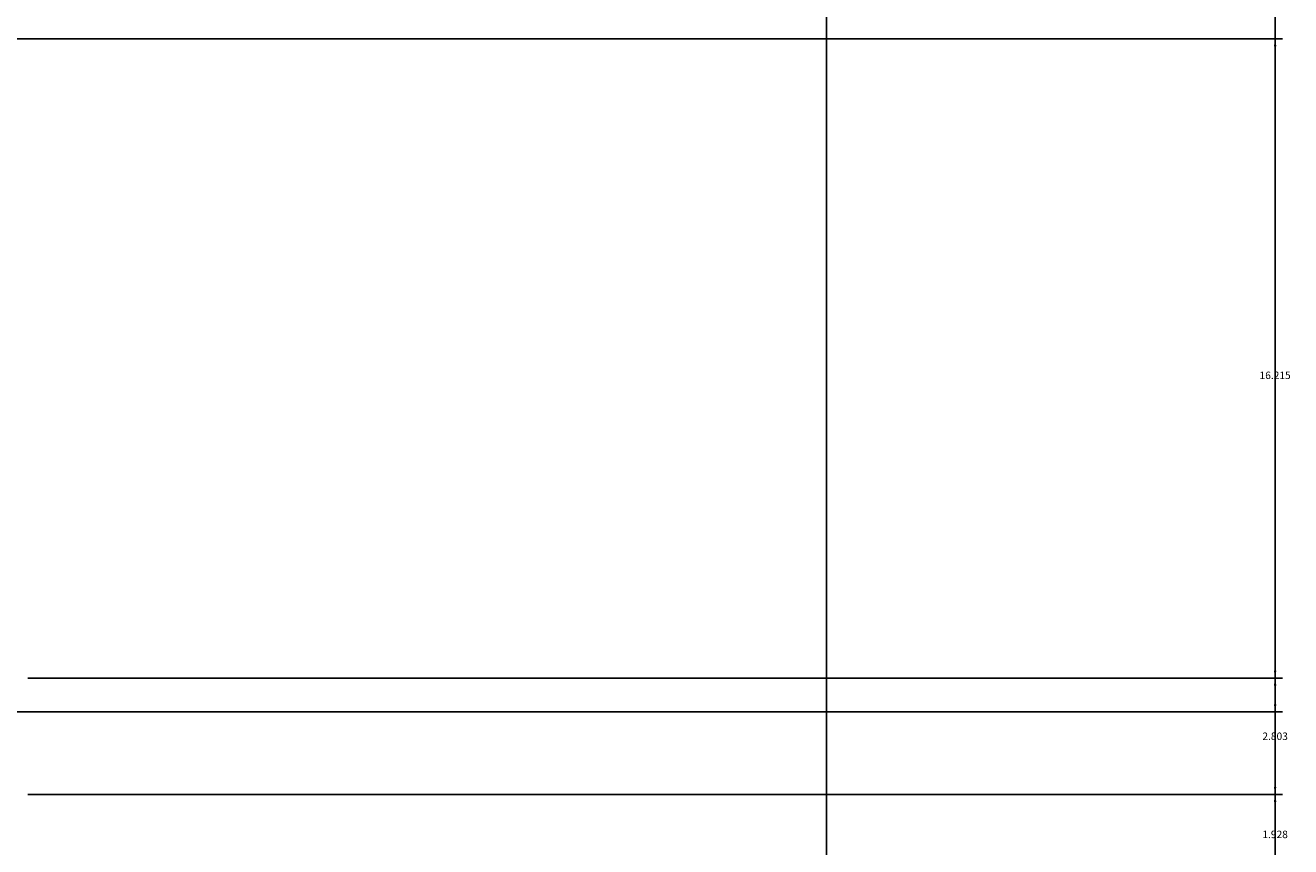
# Model space of a CAD drawing. Units: inches. Extents: x -117 to 121, y -77 to 40.
# Tile 41 of 45: x 91 to 121, y -43 to -23. Entities that reach past the tile are written whole.
import ezdxf

# ---------------------------------------------------------------- set-up
doc = ezdxf.new("R2010")
doc.units = ezdxf.units.IN
doc.header["$MEASUREMENT"] = 0
doc.layers.add('A-ANNO-DIMS', color=2, linetype='Continuous', lineweight=18)
doc.styles.get("Standard").update_dxf_attribs({"font": 'arial.ttf'})
doc.dimstyles.get("Standard").update_dxf_attribs({"dimtxt": 0.18, "dimasz": 0.18, "dimexe": 0.18, "dimexo": 0.0625, "dimgap": 0.09, "dimtad": 0, "dimtih": 1, "dimtoh": 1, "dimdec": 4, "dimzin": 0, "dimdsep": 46, "dimtxsty": 'Standard', "dimcen": 0.09, "dimadec": 0, "dimazin": 0, "dimtfac": 1, "dimtdec": 4, "dimtofl": 0, "dimtmove": 0, "dimatfit": 3, "dimfxl": 1, "dimtolj": 1, "dimtzin": 0, "dimarcsym": 0})

# ---------------------------------------------------------------- blocks, each defined once
blk = doc.blocks.new('*D14')
at = {"layer": 'A-ANNO-DIMS', "color": 0, "lineweight": -2, "transparency": 16777216}
for p, q in [((90.611, -38.902), (120.84, -38.902)), ((120.66, -39.082), (120.66, -49.957)), ((120.66, -61.196), (120.66, -50.321)), ((109.913, -61.376), (120.84, -61.376))]:
    blk.add_line(p, q, dxfattribs=at)
at = {"layer": 'A-ANNO-DIMS', "color": 0, "transparency": 16777216}
for points in [[(120.63, -39.082), (120.69, -39.082), (120.66, -38.902)], [(120.63, -61.196), (120.69, -61.196), (120.66, -61.376)]]:
    blk.add_solid(points, dxfattribs=at)
at = {"layer": 'Defpoints', "color": 0, "transparency": 16777216}
for p in [(90.549, -38.902), (109.85, -61.376), (120.66, -61.376)]:
    blk.add_point(p, dxfattribs=at)
at = {"layer": 'A-ANNO-DIMS', "color": 0, "transparency": 16777216, "insert": (120.66, -50.139), "char_height": 0.18, "attachment_point": 5}
blk.add_mtext('\\A1;22.473', dxfattribs=at)
blk = doc.blocks.new('*D15')
at = {"layer": 'A-ANNO-DIMS', "color": 0, "lineweight": -2, "transparency": 16777216}
for p, q in [((87.304, -2.653), (120.84, -2.653)), ((120.66, -2.833), (120.66, -20.595)), ((120.66, -38.722), (120.66, -20.959)), ((90.611, -38.902), (120.84, -38.902))]:
    blk.add_line(p, q, dxfattribs=at)
at = {"layer": 'A-ANNO-DIMS', "color": 0, "transparency": 16777216}
for points in [[(120.63, -2.833), (120.69, -2.833), (120.66, -2.653)], [(120.63, -38.722), (120.69, -38.722), (120.66, -38.902)]]:
    blk.add_solid(points, dxfattribs=at)
at = {"layer": 'Defpoints', "color": 0, "transparency": 16777216}
for p in [(87.242, -2.653), (90.549, -38.902), (120.66, -38.902)]:
    blk.add_point(p, dxfattribs=at)
at = {"layer": 'A-ANNO-DIMS', "color": 0, "transparency": 16777216, "insert": (120.66, -20.777), "char_height": 0.18, "attachment_point": 5}
blk.add_mtext('\\A1;36.25', dxfattribs=at)
blk = doc.blocks.new('*D24')
at = {"layer": 'A-ANNO-DIMS', "color": 0, "lineweight": -2, "transparency": 16777216}
for p, q in [((87.242, 3.166), (87.242, 38.61)), ((87.422, 38.43), (98.081, 38.43)), ((109.67, 38.43), (99.011, 38.43)), ((109.85, -61.313), (109.85, 38.61))]:
    blk.add_line(p, q, dxfattribs=at)
at = {"layer": 'A-ANNO-DIMS', "color": 0, "transparency": 16777216}
for points in [[(87.422, 38.46), (87.422, 38.4), (87.242, 38.43)], [(109.67, 38.46), (109.67, 38.4), (109.85, 38.43)]]:
    blk.add_solid(points, dxfattribs=at)
at = {"layer": 'Defpoints', "color": 0, "transparency": 16777216}
for p in [(109.85, 38.43), (87.242, 3.104), (109.85, -61.376)]:
    blk.add_point(p, dxfattribs=at)
at = {"layer": 'A-ANNO-DIMS', "color": 0, "transparency": 16777216, "insert": (98.546, 38.43), "char_height": 0.18, "attachment_point": 5}
blk.add_mtext('\\A1;22.609', dxfattribs=at)
blk = doc.blocks.new('*D35')
at = {"layer": 'A-ANNO-DIMS', "color": 0, "lineweight": -2, "transparency": 16777216}
for p, q in [((90.611, -41.705), (120.84, -41.705)), ((120.66, -41.885), (120.66, -42.487)), ((120.66, -43.453), (120.66, -42.851)), ((90.611, -43.633), (120.84, -43.633))]:
    blk.add_line(p, q, dxfattribs=at)
at = {"layer": 'A-ANNO-DIMS', "color": 0, "transparency": 16777216}
for points in [[(120.63, -41.885), (120.69, -41.885), (120.66, -41.705)], [(120.63, -43.453), (120.69, -43.453), (120.66, -43.633)]]:
    blk.add_solid(points, dxfattribs=at)
at = {"layer": 'Defpoints', "color": 0, "transparency": 16777216}
for p in [(90.549, -41.705), (120.66, -41.705), (90.549, -43.633)]:
    blk.add_point(p, dxfattribs=at)
at = {"layer": 'A-ANNO-DIMS', "color": 0, "transparency": 16777216, "insert": (120.66, -42.669), "char_height": 0.18, "attachment_point": 5}
blk.add_mtext('\\A1;1.928', dxfattribs=at)
blk = doc.blocks.new('*D36')
at = {"layer": 'A-ANNO-DIMS', "color": 0, "lineweight": -2, "transparency": 16777216}
for p, q in [((90.611, -38.902), (120.84, -38.902)), ((120.66, -39.082), (120.66, -40.122)), ((120.66, -41.525), (120.66, -40.486)), ((90.611, -41.705), (120.84, -41.705))]:
    blk.add_line(p, q, dxfattribs=at)
at = {"layer": 'A-ANNO-DIMS', "color": 0, "transparency": 16777216}
for points in [[(120.63, -39.082), (120.69, -39.082), (120.66, -38.902)], [(120.63, -41.525), (120.69, -41.525), (120.66, -41.705)]]:
    blk.add_solid(points, dxfattribs=at)
at = {"layer": 'Defpoints', "color": 0, "transparency": 16777216}
for p in [(90.549, -38.902), (120.66, -38.902), (90.549, -41.705)]:
    blk.add_point(p, dxfattribs=at)
at = {"layer": 'A-ANNO-DIMS', "color": 0, "transparency": 16777216, "insert": (120.66, -40.304), "char_height": 0.18, "attachment_point": 5}
blk.add_mtext('\\A1;2.803', dxfattribs=at)
blk = doc.blocks.new('*D49')
at = {"layer": 'A-ANNO-DIMS', "color": 0, "lineweight": -2, "transparency": 16777216}
for p, q in [((-45.422, -23.501), (120.84, -23.501)), ((120.66, -23.681), (120.66, -31.426)), ((120.66, -39.536), (120.66, -31.79)), ((-45.471, -39.716), (120.84, -39.716))]:
    blk.add_line(p, q, dxfattribs=at)
at = {"layer": 'A-ANNO-DIMS', "color": 0, "transparency": 16777216}
for points in [[(120.63, -23.681), (120.69, -23.681), (120.66, -23.501)], [(120.63, -39.536), (120.69, -39.536), (120.66, -39.716)]]:
    blk.add_solid(points, dxfattribs=at)
at = {"layer": 'Defpoints', "color": 0, "transparency": 16777216}
for p in [(-45.485, -23.501), (120.66, -23.501), (-45.533, -39.716)]:
    blk.add_point(p, dxfattribs=at)
at = {"layer": 'A-ANNO-DIMS', "color": 0, "transparency": 16777216, "insert": (120.66, -31.608), "char_height": 0.18, "attachment_point": 5}
blk.add_mtext('\\A1;16.215', dxfattribs=at)

msp = doc.modelspace()

# ---------------------------------------------------------------- dimensions: what is measured, and where the dimension line sits
at = {"layer": 'A-ANNO-DIMS'}
dim = msp.add_linear_dim(base=(109.8502, 38.4297), p1=(87.2416, 3.1036), p2=(109.8502, -61.3756), dimstyle='Standard', override={"dimdec": 3, "dimlfac": 1, "dimrnd": 0, "dimzin": 0, "dimdsep": 46, "dimlunit": 2}, dxfattribs=at)
dim.commit()
dim.dimension.update_dxf_attribs({"geometry": '*D24', "text_midpoint": (98.5459, 38.4297)})
for base, p1, p2, override, picture, middle in [((120.6602, -38.9022), (87.2416, -2.6528), (90.5486, -38.9022), {"dimdec": 2, "dimlfac": 1, "dimrnd": 0, "dimzin": 0, "dimdsep": 46, "dimlunit": 2}, '*D15', (120.6602, -20.7775)), ((120.6602, -23.5007), (-45.5331, -39.716), (-45.4848, -23.5007), {"dimdec": 3, "dimlfac": 1, "dimrnd": 0, "dimzin": 0, "dimdsep": 46, "dimlunit": 2}, '*D49', (120.6602, -31.6083)), ((120.6602, -61.3756), (90.5486, -38.9022), (109.8502, -61.3756), {"dimdec": 3, "dimlfac": 1, "dimrnd": 0, "dimzin": 0, "dimdsep": 46, "dimlunit": 2}, '*D14', (120.6602, -50.1389)), ((120.6602, -38.9022), (90.5486, -41.7053), (90.5486, -38.9022), {"dimdec": 3, "dimlfac": 1, "dimrnd": 0, "dimzin": 0, "dimdsep": 46, "dimlunit": 2}, '*D36', (120.6602, -40.3038)), ((120.6602, -41.7053), (90.5486, -43.6334), (90.5486, -41.7053), {"dimdec": 3, "dimlfac": 1, "dimrnd": 0, "dimzin": 0, "dimdsep": 46, "dimlunit": 2}, '*D35', (120.6602, -42.6693))]:
    dim = msp.add_linear_dim(base=base, p1=p1, p2=p2, angle=90, dimstyle='Standard', override=override, dxfattribs=at)
    dim.commit()
    dim.dimension.update_dxf_attribs({"geometry": picture, "text_midpoint": middle})

doc.saveas('drawing.dxf')
